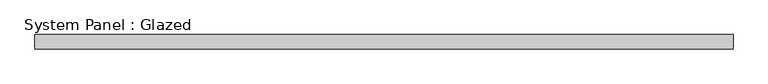
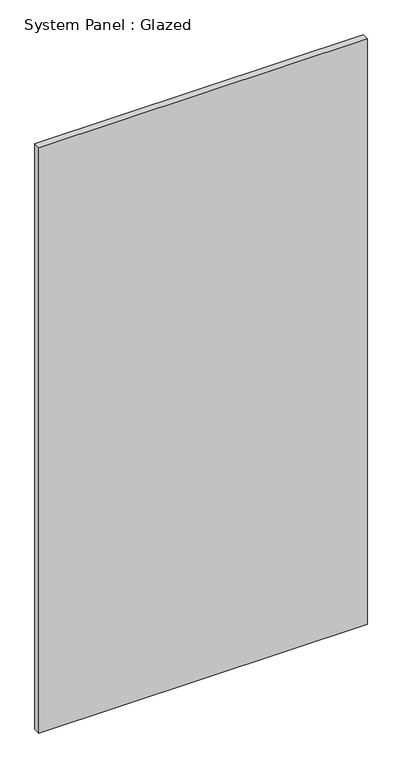
"""IFC4 building model written with IfcOpenShell, lengths in millimetres: plate geometry, System Panel : Glazed."""

from ifc_helpers import new_model, si_unit, origin, origin_with_axes, place, context, project, spatial, polyline, outline, extrude, source, transform, mapped, element, save


def system_panel_glazed_e6f1e35b(model_context):
    return source(origin(), model_context, "Body", "SweptSolid", [
        extrude(outline(polyline([(622.3, 19.05), (-622.3, 19.05), (-622.3, 44.45), (622.3, 44.45), (622.3, 19.05)])), origin_with_axes(), (0.0, 0.0, 1.0), 2343.15),
    ])


if __name__ == "__main__":
    model = new_model("IFC4")
    model_context = context("Model", 3, world=origin())
    ifc_project = project(units=[si_unit("LENGTHUNIT", "METRE", prefix="MILLI")], contexts=[model_context])
    site = spatial("IfcSite", under=ifc_project)
    building = spatial("IfcBuilding", under=site)
    placement = place(None, origin())
    system_panel_glazed_shape = system_panel_glazed_e6f1e35b(model_context)
    element("IfcPlate", 1, ObjectType="System Panel : Glazed", at=placement, inside=building, context=model_context, shape_type="MappedRepresentation", body=[
        mapped(system_panel_glazed_shape, transform((0.0, 0.0, 0.0), x_axis=(1.0, 0.0, 0.0), y_axis=(0.0, 1.0, 0.0), z_axis=(0.0, 0.0, 1.0))),
    ])
    save(model, "model.ifc")

# Revit data of these elements
# Type "System Panel : Glazed"
#   Construction Type Id = "GSP4R"
#   Analytic Construction = "1/8 in Pilkington single glazing"
#   Visual Light Transmittance = 0.9
#   Solar Heat Gain Coefficient = 0.86
#   Heat Transfer Coefficient (U) = 1.18115 BTU/(h·ft²·°F)
#   Define Thermal Properties by = 1
# Element 1 (IfcPlate, "System Panel : Glazed")
#   Materials on its faces: "Glass"
# Materials
#   "Glass": class "Glass", colour RGB 0 128 192, transparency 0.75, Description = "Soda Lime Glass", Cost = 0
